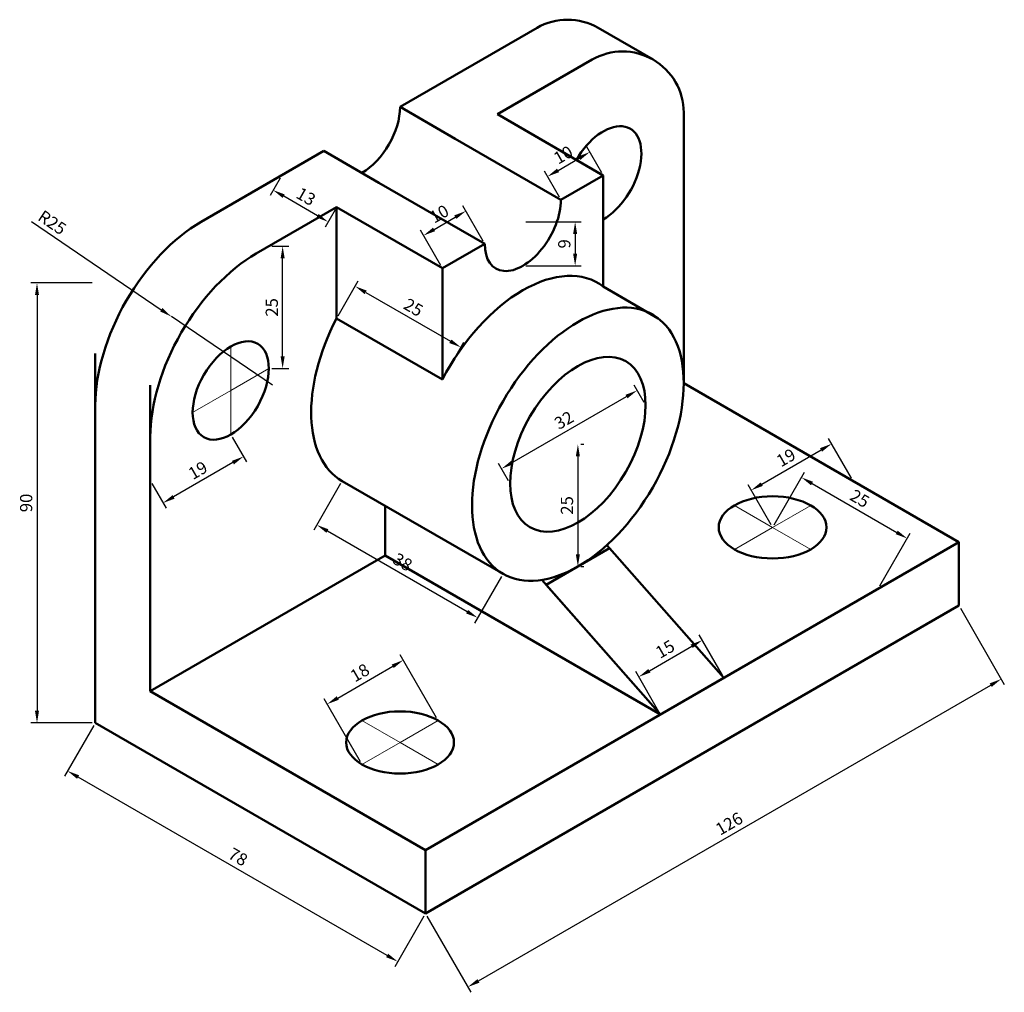
# Model space of a CAD drawing. Units: millimetres. Extents: x 14 to 216, y 199 to 398.
import ezdxf

# ---------------------------------------------------------------- set-up
doc = ezdxf.new("R2010")
doc.units = ezdxf.units.MM
doc.linetypes.add('CENTER', pattern=[50.8, 31.75, -6.35, 6.35, -6.35])
for name, color, linetype, lineweight in [('M-CNTR', 1, 'CENTER', 18), ('M-DIMS', 2, 'Continuous', 25), ('M-OUTL', 7, 'Continuous', 50)]:
    doc.layers.add(name, color=color, linetype=linetype, lineweight=lineweight)
doc.styles.get("Standard").update_dxf_attribs({"font": 'arial.ttf'})
doc.dimstyles.new('ISO-25', dxfattribs={"dimtxt": 2.5, "dimasz": 2.5, "dimexe": 1.25, "dimexo": 0.625, "dimtad": 1, "dimtxsty": 'Standard', "dimcen": 2.5, "dimadec": 0, "dimazin": 0, "dimtfac": 1, "dimtmove": 0, "dimatfit": 3, "dimfxl": 1, "dimarcsym": 0})

# ---------------------------------------------------------------- blocks, each defined once
blk = doc.blocks.new('*D1')
at = {"layer": 'Defpoints', "color": 0, "transparency": 16777216}
for p in [(206.54, 277.84), (215.21, 262.82), (97.42, 214.84)]:
    blk.add_point(p, dxfattribs=at)
at = {"layer": 'M-DIMS', "color": 0, "lineweight": -2, "transparency": 16777216}
for p, q in [((206.85, 277.3), (215.84, 261.73)), ((108.26, 201.07), (213.05, 261.57)), ((97.73, 214.3), (106.72, 198.73))]:
    blk.add_line(p, q, dxfattribs=at)
at = {"layer": 'M-DIMS', "color": 0, "transparency": 16777216}
for points in [[(212.84, 261.93), (213.26, 261.21), (215.21, 262.82)], [(108.05, 201.43), (108.47, 200.71), (106.09, 199.82)]]:
    blk.add_solid(points, dxfattribs=at)
at = {"layer": 'M-DIMS', "color": 0, "transparency": 16777216, "insert": (159.7, 232.96), "char_height": 2.5, "attachment_point": 5, "rotation": 30}
blk.add_mtext('126', dxfattribs=at)
blk = doc.blocks.new('*D2')
at = {"layer": 'Defpoints', "color": 0, "transparency": 16777216}
for p in [(29.87, 253.84), (24.2, 244.01), (97.42, 214.84)]:
    blk.add_point(p, dxfattribs=at)
at = {"layer": 'M-DIMS', "color": 0, "lineweight": -2, "transparency": 16777216}
for p, q in [((29.56, 253.3), (23.57, 242.93)), ((89.58, 206.26), (26.36, 242.76)), ((97.11, 214.3), (91.12, 203.93))]:
    blk.add_line(p, q, dxfattribs=at)
at = {"layer": 'M-DIMS', "color": 0, "transparency": 16777216}
for points in [[(26.57, 243.12), (26.15, 242.4), (24.2, 244.01)], [(89.79, 206.62), (89.37, 205.9), (91.75, 205.01)]]:
    blk.add_solid(points, dxfattribs=at)
at = {"layer": 'M-DIMS', "color": 0, "transparency": 16777216, "insert": (58.92, 226.16), "char_height": 2.5, "attachment_point": 5, "rotation": 330}
blk.add_mtext('78', dxfattribs=at)
blk = doc.blocks.new('*D3')
at = {"layer": 'Defpoints', "color": 0, "transparency": 16777216}
for p in [(29.87, 343.84), (17.95, 253.84), (29.87, 253.84)]:
    blk.add_point(p, dxfattribs=at)
at = {"layer": 'M-DIMS', "color": 0, "lineweight": -2, "transparency": 16777216}
for p, q in [((29.24, 343.84), (16.7, 343.84)), ((17.95, 341.34), (17.95, 256.34)), ((29.24, 253.84), (16.7, 253.84))]:
    blk.add_line(p, q, dxfattribs=at)
at = {"layer": 'M-DIMS', "color": 0, "transparency": 16777216}
for points in [[(17.53, 341.34), (18.36, 341.34), (17.95, 343.84)], [(17.53, 256.34), (18.36, 256.34), (17.95, 253.84)]]:
    blk.add_solid(points, dxfattribs=at)
at = {"layer": 'M-DIMS', "color": 0, "transparency": 16777216, "insert": (16.05, 298.84), "char_height": 2.5, "attachment_point": 5, "rotation": 90}
blk.add_mtext('90', dxfattribs=at)
blk = doc.blocks.new('*D4')
at = {"layer": 'Defpoints', "color": 0, "transparency": 16777216}
for p in [(67.97, 365.84), (66.24, 362.84), (79.23, 359.34)]:
    blk.add_point(p, dxfattribs=at)
at = {"layer": 'M-DIMS', "color": 0, "lineweight": -2, "transparency": 16777216}
for p, q in [((67.66, 365.3), (65.62, 361.76)), ((75.34, 357.59), (68.41, 361.59)), ((78.92, 358.8), (76.88, 355.26))]:
    blk.add_line(p, q, dxfattribs=at)
at = {"layer": 'M-DIMS', "color": 0, "transparency": 16777216}
for points in [[(68.62, 361.95), (68.2, 361.23), (66.24, 362.84)], [(75.55, 357.95), (75.13, 357.23), (77.5, 356.34)]]:
    blk.add_solid(points, dxfattribs=at)
at = {"layer": 'M-DIMS', "color": 0, "transparency": 16777216, "insert": (72.82, 361.24), "char_height": 2.5, "attachment_point": 5, "rotation": 330}
blk.add_mtext('13', dxfattribs=at)
blk = doc.blocks.new('*D5')
at = {"layer": 'Defpoints', "color": 0, "transparency": 16777216}
for p in [(65.38, 351.34), (68.2, 351.34), (65.38, 326.34)]:
    blk.add_point(p, dxfattribs=at)
at = {"layer": 'M-DIMS', "color": 0, "lineweight": -2, "transparency": 16777216}
for p, q in [((66, 351.34), (69.45, 351.34)), ((68.2, 328.84), (68.2, 348.84)), ((66, 326.34), (69.45, 326.34))]:
    blk.add_line(p, q, dxfattribs=at)
at = {"layer": 'M-DIMS', "color": 0, "transparency": 16777216}
for points in [[(67.78, 348.84), (68.62, 348.84), (68.2, 351.34)], [(67.78, 328.84), (68.62, 328.84), (68.2, 326.34)]]:
    blk.add_solid(points, dxfattribs=at)
at = {"layer": 'M-DIMS', "color": 0, "transparency": 16777216, "insert": (66.3, 338.84), "char_height": 2.5, "attachment_point": 5, "rotation": 90}
blk.add_mtext('25', dxfattribs=at)
blk = doc.blocks.new('*D6')
at = {"layer": 'Defpoints', "color": 0, "transparency": 16777216}
for p in [(57.58, 312.84), (41.13, 303.34), (43.73, 298.83)]:
    blk.add_point(p, dxfattribs=at)
at = {"layer": 'M-DIMS', "color": 0, "lineweight": -2, "transparency": 16777216}
for p, q in [((57.89, 312.3), (60.81, 307.25)), ((58.02, 307.08), (45.9, 300.08)), ((41.44, 302.8), (44.36, 297.75))]:
    blk.add_line(p, q, dxfattribs=at)
at = {"layer": 'M-DIMS', "color": 0, "transparency": 16777216}
for points in [[(57.81, 307.44), (58.23, 306.72), (60.19, 308.33)], [(45.69, 300.44), (46.1, 299.72), (43.73, 298.83)]]:
    blk.add_solid(points, dxfattribs=at)
at = {"layer": 'M-DIMS', "color": 0, "transparency": 16777216, "insert": (51.01, 305.23), "char_height": 2.5, "attachment_point": 5, "rotation": 30}
blk.add_mtext('19', dxfattribs=at)
blk = doc.blocks.new('*D7')
at = {"layer": 'Defpoints', "color": 0, "transparency": 16777216}
for p in [(117.34, 356.34), (117.34, 347.34), (128.04, 347.34)]:
    blk.add_point(p, dxfattribs=at)
at = {"layer": 'M-DIMS', "color": 0, "lineweight": -2, "transparency": 16777216}
for p, q in [((117.96, 356.34), (129.29, 356.34)), ((128.04, 353.84), (128.04, 349.84)), ((117.96, 347.34), (129.29, 347.34))]:
    blk.add_line(p, q, dxfattribs=at)
at = {"layer": 'M-DIMS', "color": 0, "transparency": 16777216}
for points in [[(127.62, 353.84), (128.46, 353.84), (128.04, 356.34)], [(127.62, 349.84), (128.46, 349.84), (128.04, 347.34)]]:
    blk.add_solid(points, dxfattribs=at)
at = {"layer": 'M-DIMS', "color": 0, "transparency": 16777216, "insert": (126.14, 351.84), "char_height": 2.5, "attachment_point": 5, "rotation": 90}
blk.add_mtext('9', dxfattribs=at)
blk = doc.blocks.new('*D8')
at = {"layer": 'Defpoints', "color": 0, "transparency": 16777216}
for p in [(79.23, 336.59), (104.68, 330.66), (100.88, 324.09)]:
    blk.add_point(p, dxfattribs=at)
at = {"layer": 'M-DIMS', "color": 0, "lineweight": -2, "transparency": 16777216}
for p, q in [((79.55, 337.13), (83.65, 344.24)), ((85.19, 341.91), (102.51, 331.91)), ((101.2, 324.63), (105.3, 331.74))]:
    blk.add_line(p, q, dxfattribs=at)
at = {"layer": 'M-DIMS', "color": 0, "transparency": 16777216}
for points in [[(85.4, 342.27), (84.98, 341.55), (83.03, 343.16)], [(102.72, 332.27), (102.3, 331.55), (104.68, 330.66)]]:
    blk.add_solid(points, dxfattribs=at)
at = {"layer": 'M-DIMS', "color": 0, "transparency": 16777216, "insert": (94.8, 338.56), "char_height": 2.5, "attachment_point": 5, "rotation": 330}
blk.add_mtext('25', dxfattribs=at)
blk = doc.blocks.new('*D9')
at = {"layer": 'Defpoints', "color": 0, "transparency": 16777216}
for p in [(131.04, 370.61), (133.79, 365.84), (125.13, 360.84)]:
    blk.add_point(p, dxfattribs=at)
at = {"layer": 'M-DIMS', "color": 0, "lineweight": -2, "transparency": 16777216}
for p, q in [((133.48, 366.38), (130.41, 371.69)), ((124.54, 366.86), (128.87, 369.36)), ((124.82, 361.38), (121.75, 366.69))]:
    blk.add_line(p, q, dxfattribs=at)
at = {"layer": 'M-DIMS', "color": 0, "transparency": 16777216}
for points in [[(128.66, 369.72), (129.08, 369), (131.04, 370.61)], [(124.33, 367.22), (124.75, 366.5), (122.38, 365.61)]]:
    blk.add_solid(points, dxfattribs=at)
at = {"layer": 'M-DIMS', "color": 0, "transparency": 16777216, "insert": (125.76, 369.76), "char_height": 2.5, "attachment_point": 5, "rotation": 30}
blk.add_mtext('10', dxfattribs=at)
blk = doc.blocks.new('*D10')
at = {"layer": 'Defpoints', "color": 0, "transparency": 16777216}
for p in [(105.68, 358.54), (109.54, 351.84), (100.88, 346.84)]:
    blk.add_point(p, dxfattribs=at)
at = {"layer": 'M-DIMS', "color": 0, "lineweight": -2, "transparency": 16777216}
for p, q in [((109.23, 352.38), (105.05, 359.62)), ((99.18, 354.79), (103.51, 357.29)), ((100.57, 347.38), (96.39, 354.62))]:
    blk.add_line(p, q, dxfattribs=at)
at = {"layer": 'M-DIMS', "color": 0, "transparency": 16777216}
for points in [[(103.3, 357.65), (103.72, 356.93), (105.68, 358.54)], [(98.97, 355.15), (99.39, 354.43), (97.01, 353.54)]]:
    blk.add_solid(points, dxfattribs=at)
at = {"layer": 'M-DIMS', "color": 0, "transparency": 16777216, "insert": (100.39, 357.69), "char_height": 2.5, "attachment_point": 5, "rotation": 30}
blk.add_mtext('10', dxfattribs=at)
blk = doc.blocks.new('*D11')
at = {"layer": 'Defpoints', "color": 0, "transparency": 16777216}
for p in [(92.89, 266.68), (100.02, 254.34), (84.43, 245.34)]:
    blk.add_point(p, dxfattribs=at)
at = {"layer": 'M-DIMS', "color": 0, "lineweight": -2, "transparency": 16777216}
for p, q in [((99.71, 254.88), (92.27, 267.76)), ((79.47, 258.93), (90.73, 265.43)), ((84.12, 245.88), (76.68, 258.76))]:
    blk.add_line(p, q, dxfattribs=at)
at = {"layer": 'M-DIMS', "color": 0, "transparency": 16777216}
for points in [[(90.52, 265.79), (90.93, 265.07), (92.89, 266.68)], [(79.26, 259.29), (79.68, 258.57), (77.3, 257.68)]]:
    blk.add_solid(points, dxfattribs=at)
at = {"layer": 'M-DIMS', "color": 0, "transparency": 16777216, "insert": (84.15, 263.83), "char_height": 2.5, "attachment_point": 5, "rotation": 30}
blk.add_mtext('18', dxfattribs=at)
blk = doc.blocks.new('*D12')
at = {"layer": 'Defpoints', "color": 0, "transparency": 16777216}
for p in [(168.43, 293.84), (195.99, 291.56), (190.08, 281.34)]:
    blk.add_point(p, dxfattribs=at)
at = {"layer": 'M-DIMS', "color": 0, "lineweight": -2, "transparency": 16777216}
for p, q in [((168.75, 294.38), (174.96, 305.14)), ((176.5, 302.81), (193.82, 292.81)), ((190.4, 281.88), (196.61, 292.64))]:
    blk.add_line(p, q, dxfattribs=at)
at = {"layer": 'M-DIMS', "color": 0, "transparency": 16777216}
for points in [[(176.71, 303.17), (176.29, 302.45), (174.34, 304.06)], [(194.03, 293.17), (193.61, 292.45), (195.99, 291.56)]]:
    blk.add_solid(points, dxfattribs=at)
at = {"layer": 'M-DIMS', "color": 0, "transparency": 16777216, "insert": (186.11, 299.46), "char_height": 2.5, "attachment_point": 5, "rotation": 330}
blk.add_mtext('25', dxfattribs=at)
blk = doc.blocks.new('*D13')
at = {"layer": 'Defpoints', "color": 0, "transparency": 16777216}
for p in [(180.51, 310.93), (184.89, 303.34), (168.43, 293.84)]:
    blk.add_point(p, dxfattribs=at)
at = {"layer": 'M-DIMS', "color": 0, "lineweight": -2, "transparency": 16777216}
for p, q in [((184.58, 303.88), (179.88, 312.01)), ((166.22, 302.68), (178.34, 309.68)), ((168.12, 294.38), (163.43, 302.51))]:
    blk.add_line(p, q, dxfattribs=at)
at = {"layer": 'M-DIMS', "color": 0, "transparency": 16777216}
for points in [[(178.13, 310.04), (178.55, 309.32), (180.51, 310.93)], [(166.01, 303.04), (166.42, 302.32), (164.05, 301.43)]]:
    blk.add_solid(points, dxfattribs=at)
at = {"layer": 'M-DIMS', "color": 0, "transparency": 16777216, "insert": (171.33, 307.83), "char_height": 2.5, "attachment_point": 5, "rotation": 30}
blk.add_mtext('19', dxfattribs=at)
blk = doc.blocks.new('*D14')
at = {"layer": 'Defpoints', "color": 0, "transparency": 16777216}
for p in [(128.6, 310.84), (128.6, 285.84), (128.6, 285.84)]:
    blk.add_point(p, dxfattribs=at)
at = {"layer": 'M-DIMS', "color": 0, "lineweight": -2, "transparency": 16777216}
for p, q in [((129.22, 310.84), (129.85, 310.84)), ((128.6, 308.34), (128.6, 288.34)), ((129.22, 285.84), (129.85, 285.84))]:
    blk.add_line(p, q, dxfattribs=at)
at = {"layer": 'M-DIMS', "color": 0, "transparency": 16777216}
for points in [[(128.18, 308.34), (129.01, 308.34), (128.6, 310.84)], [(128.18, 288.34), (129.01, 288.34), (128.6, 285.84)]]:
    blk.add_solid(points, dxfattribs=at)
at = {"layer": 'M-DIMS', "color": 0, "transparency": 16777216, "insert": (126.69, 298.34), "char_height": 2.5, "attachment_point": 5, "rotation": 90}
blk.add_mtext('25', dxfattribs=at)
blk = doc.blocks.new('*D15')
at = {"layer": 'Defpoints', "color": 0, "transparency": 16777216}
for p in [(140.72, 321.85), (142.45, 318.84), (114.74, 302.84)]:
    blk.add_point(p, dxfattribs=at)
at = {"layer": 'M-DIMS', "color": 0, "lineweight": -2, "transparency": 16777216}
for p, q in [((142.14, 319.38), (140.09, 322.93)), ((115.17, 307.1), (138.55, 320.6)), ((114.43, 303.38), (112.38, 306.93))]:
    blk.add_line(p, q, dxfattribs=at)
at = {"layer": 'M-DIMS', "color": 0, "transparency": 16777216}
for points in [[(138.34, 320.96), (138.76, 320.24), (140.72, 321.85)], [(114.96, 307.46), (115.38, 306.74), (113, 305.85)]]:
    blk.add_solid(points, dxfattribs=at)
at = {"layer": 'M-DIMS', "color": 0, "transparency": 16777216, "insert": (125.91, 315.49), "char_height": 2.5, "attachment_point": 5, "rotation": 30}
blk.add_mtext('32', dxfattribs=at)
blk = doc.blocks.new('*D16')
at = {"layer": 'Defpoints', "color": 0, "transparency": 16777216}
for p in [(45.44, 336.95), (66.13, 322.91)]:
    blk.add_point(p, dxfattribs=at)
at = {"layer": 'M-DIMS', "color": 0, "lineweight": -2, "transparency": 16777216}
for p, q in [((16.81, 356.39), (43.38, 338.35)), ((66.13, 322.91), (45.44, 336.95))]:
    blk.add_line(p, q, dxfattribs=at)
at = {"layer": 'M-DIMS', "color": 0, "transparency": 16777216}
blk.add_solid([(43.61, 338.7), (43.14, 338.01), (45.44, 336.95)], dxfattribs=at)
at = {"layer": 'M-DIMS', "color": 0, "transparency": 16777216, "insert": (20.88, 355.93), "char_height": 2.5, "attachment_point": 5, "rotation": 325.8245}
blk.add_mtext('R25', dxfattribs=at)
blk = doc.blocks.new('*D17')
at = {"layer": 'Defpoints', "color": 0, "transparency": 16777216}
for p in [(154.04, 270.76), (158.47, 263.09), (145.48, 255.59)]:
    blk.add_point(p, dxfattribs=at)
at = {"layer": 'M-DIMS', "color": 0, "lineweight": -2, "transparency": 16777216}
for p, q in [((158.16, 263.63), (153.42, 271.85)), ((143.22, 264.51), (151.88, 269.51)), ((145.17, 256.13), (140.43, 264.35))]:
    blk.add_line(p, q, dxfattribs=at)
at = {"layer": 'M-DIMS', "color": 0, "transparency": 16777216}
for points in [[(151.67, 269.87), (152.09, 269.15), (154.04, 270.76)], [(143.01, 264.87), (143.43, 264.15), (141.05, 263.26)]]:
    blk.add_solid(points, dxfattribs=at)
at = {"layer": 'M-DIMS', "color": 0, "transparency": 16777216, "insert": (146.6, 268.66), "char_height": 2.5, "attachment_point": 5, "rotation": 30}
blk.add_mtext('15', dxfattribs=at)
blk = doc.blocks.new('*D18')
at = {"layer": 'Defpoints', "color": 0, "transparency": 16777216}
for p in [(80.38, 303.32), (75.19, 294.34), (113.29, 284.32)]:
    blk.add_point(p, dxfattribs=at)
at = {"layer": 'M-DIMS', "color": 0, "lineweight": -2, "transparency": 16777216}
for p, q in [((80.07, 302.78), (74.56, 293.25)), ((105.93, 276.59), (77.35, 293.09)), ((112.97, 283.78), (107.47, 274.25))]:
    blk.add_line(p, q, dxfattribs=at)
at = {"layer": 'M-DIMS', "color": 0, "transparency": 16777216}
for points in [[(77.56, 293.45), (77.15, 292.73), (75.19, 294.34)], [(106.14, 276.95), (105.73, 276.23), (108.1, 275.34)]]:
    blk.add_solid(points, dxfattribs=at)
at = {"layer": 'M-DIMS', "color": 0, "transparency": 16777216, "insert": (92.6, 286.48), "char_height": 2.5, "attachment_point": 5, "rotation": 330}
blk.add_mtext('38', dxfattribs=at)

msp = doc.modelspace()

# ---------------------------------------------------------------- linework, layer by layer
at = {"layer": 'M-CNTR'}
for p, q in [((57.582, 321.839), (57.582, 330.839)), ((57.582, 321.839), (65.377, 326.339)), ((57.582, 321.839), (49.788, 317.339)), ((57.582, 321.839), (57.582, 312.839)), ((168.434, 293.839), (160.639, 298.339)), ((168.434, 293.839), (176.228, 298.339)), ((168.434, 293.839), (160.639, 289.339)), ((168.434, 293.839), (176.228, 289.339)), ((92.223, 249.839), (84.429, 254.339)), ((92.223, 249.839), (100.018, 254.339)), ((92.223, 249.839), (84.429, 245.339)), ((92.223, 249.839), (100.018, 245.339))]:
    msp.add_line(p, q, dxfattribs=at)
at = {"layer": 'M-OUTL'}
for p, q in [((92.223, 379.839), (120.239, 396.014)), ((132.739, 396.014), (143.997, 389.514)), ((112.142, 378.339), (131.497, 389.514)), ((131.497, 389.514), (112.142, 378.339)), ((103.482, 373.339), (92.223, 379.839)), ((133.793, 365.839), (112.142, 378.339)), ((150.247, 323.339), (150.247, 378.689)), ((125.132, 360.839), (103.482, 373.339)), ((76.635, 370.839), (51.52, 356.339)), ((87.893, 364.339), (76.635, 370.839)), ((125.132, 360.839), (133.793, 365.839)), ((133.793, 365.839), (133.793, 343.087)), ((109.544, 351.839), (87.893, 364.339)), ((125.132, 360.839), (125.132, 360.839)), ((79.233, 359.339), (62.778, 349.839)), ((100.884, 346.839), (79.233, 359.339)), ((79.233, 359.339), (79.233, 336.587)), ((109.544, 351.839), (100.884, 346.839)), ((100.884, 346.839), (100.884, 324.087)), ((133.793, 343.087), (145.051, 336.587)), ((100.884, 324.087), (79.233, 336.587)), ((29.87, 253.839), (29.87, 329.406)), ((29.87, 253.839), (29.87, 329.406)), ((29.87, 253.839), (29.87, 329.406)), ((41.128, 260.339), (41.128, 322.906)), ((206.539, 290.839), (150.247, 323.339)), ((150.247, 323.339), (150.247, 323.339)), ((113.287, 284.323), (80.378, 303.323)), ((89.192, 288.089), (89.192, 298.234)), ((206.539, 290.839), (97.42, 227.839)), ((135.092, 289.589), (134.532, 290.224)), ((206.539, 277.839), (206.539, 290.839)), ((41.128, 260.339), (89.192, 288.089)), ((145.484, 255.589), (89.192, 288.089)), ((135.092, 289.589), (122.101, 282.089)), ((135.092, 289.589), (158.474, 263.089)), ((145.484, 255.589), (121.229, 283.078)), ((122.101, 282.089), (145.484, 255.589)), ((97.42, 214.839), (206.539, 277.839)), ((151.979, 259.339), (158.474, 263.089)), ((97.42, 227.839), (41.128, 260.339)), ((97.42, 227.839), (151.979, 259.339)), ((97.42, 214.839), (29.87, 253.839)), ((97.42, 227.839), (97.42, 214.839))]:
    msp.add_line(p, q, dxfattribs=at)
for centre, start in [((126.489, 385.189), 60), ((137.747, 378.689), 0)]:
    msp.add_arc(centre, 12.5, start, 120, dxfattribs=at)
for centre, major_axis, start_param, end_param in [((84.429, 375.339), (5.511, 9.546), 3.9269908, 5.4977871), ((133.793, 365.839), (-5.511, -9.546), 7.0685835, 10.9955743), ((117.338, 356.339), (-5.511, -9.546), 5.4977871, 8.6393798), ((51.52, 331.339), (-15.309, -26.516), 3.9269867, 5.4977913), ((62.778, 324.839), (-15.309, -26.516), 3.9269867, 5.4977913), ((117.338, 317.339), (-15.309, -26.517), 9.346863, 11.0734892), ((95.687, 329.839), (-15.309, -26.517), 4.7903039, 6.2831853)]:
    msp.add_ellipse(centre, major_axis=major_axis, ratio=0.5773503, start_param=start_param, end_param=end_param, dxfattribs=at)
for centre, major_axis in [((128.596, 310.839), (-15.309, -26.517)), ((57.582, 321.839), (-5.511, -9.546)), ((128.596, 310.839), (-9.798, -16.971)), ((168.434, 293.839), (-11.023, 0)), ((92.223, 249.839), (-11.023, 0))]:
    msp.add_ellipse(centre, major_axis=major_axis, ratio=0.5773503, dxfattribs=at)

# ---------------------------------------------------------------- dimensions: what is measured, and where the dimension line sits
at = {"layer": 'M-DIMS'}
for p1, p2, distance, picture, middle in [((125.132, 360.839), (133.793, 365.839), 5.511, '*D9', (125.756, 369.759)), ((79.233, 359.339), (67.975, 365.839), 3.46, '*D4', (72.825, 361.24)), ((100.884, 346.839), (109.544, 351.839), 7.738, '*D10', (100.394, 357.687)), ((79.233, 336.587), (100.884, 324.087), 7.589, '*D8', (94.803, 338.556)), ((114.74, 302.839), (142.453, 318.839), 3.472, '*D15', (125.909, 315.494)), ((57.582, 312.839), (41.128, 303.339), 5.205, '*D6', (51.007, 305.228)), ((168.434, 293.839), (184.888, 303.339), 8.765, '*D13', (171.328, 307.827)), ((168.434, 293.839), (190.084, 281.339), 11.804, '*D12', (186.112, 299.459)), ((113.287, 284.323), (80.378, 303.323), 10.377, '*D18', (92.595, 286.484)), ((97.42, 214.839), (206.539, 277.839), -17.347, '*D1', (159.702, 232.963)), ((145.484, 255.589), (158.474, 263.089), 8.861, '*D17', (146.598, 268.66)), ((84.429, 245.339), (100.018, 254.339), 14.252, '*D11', (84.147, 263.829)), ((97.42, 214.839), (29.87, 253.839), 11.346, '*D2', (58.922, 226.16))]:
    dim = msp.add_aligned_dim(p1=p1, p2=p2, distance=distance, dimstyle='ISO-25', override={"dimclrd": 0, "dimclre": 0, "dimclrt": 0}, dxfattribs=at)
    dim.commit()
    dim.dimension.update_dxf_attribs({"geometry": picture, "text_midpoint": middle})
dim = msp.add_radius_dim(center=(66.128, 322.906), mpoint=(45.445, 336.949), dimstyle='ISO-25', override={"dimclrd": 0, "dimclre": 0, "dimclrt": 0}, dxfattribs=at)
dim.commit()
dim.dimension.update_dxf_attribs({"geometry": '*D16', "text_midpoint": (19.809, 354.355), "dimtype": 164})
for base, p1, p2, picture, middle in [((128.039, 347.339), (117.338, 356.339), (117.338, 347.339), '*D7', (126.138, 351.839)), ((68.201, 351.339), (65.377, 326.339), (65.377, 351.339), '*D5', (66.3, 338.839)), ((17.948, 253.839), (29.87, 343.839), (29.87, 253.839), '*D3', (16.047, 298.839)), ((128.596, 285.839), (128.596, 310.839), (128.596, 285.839), '*D14', (126.695, 298.339))]:
    dim = msp.add_linear_dim(base=base, p1=p1, p2=p2, angle=90, dimstyle='ISO-25', override={"dimclrd": 0, "dimclre": 0, "dimclrt": 0}, dxfattribs=at)
    dim.commit()
    dim.dimension.update_dxf_attribs({"geometry": picture, "text_midpoint": middle})

doc.saveas('drawing.dxf')
